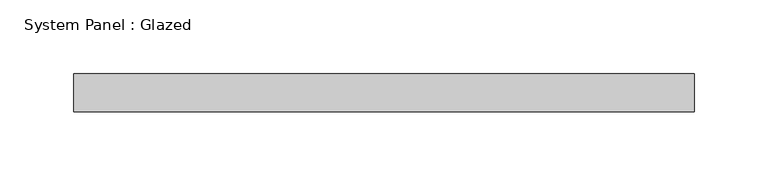
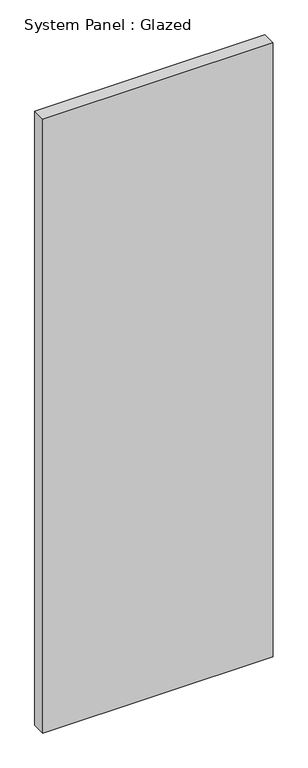
"""IFC4 building model written with IfcOpenShell, lengths in millimetres: plate geometry, System Panel : Glazed."""

from ifc_helpers import new_model, si_unit, origin, origin_with_axes, place, context, project, spatial, polyline, outline, extrude, source, transform, mapped, element, save


def system_panel_glazed_75a4b6fa(model_context):
    return source(origin(), model_context, "Body", "SweptSolid", [
        extrude(outline(polyline([(209.55, 19.05), (-209.55, 19.05), (-209.55, 44.45), (209.55, 44.45), (209.55, 19.05)])), origin_with_axes(), (0.0, 0.0, 1.0), 1181.1),
    ])


if __name__ == "__main__":
    model = new_model("IFC4")
    model_context = context("Model", 3, world=origin())
    ifc_project = project(units=[si_unit("LENGTHUNIT", "METRE", prefix="MILLI")], contexts=[model_context])
    site = spatial("IfcSite", under=ifc_project)
    building = spatial("IfcBuilding", under=site)
    placement = place(None, origin())
    system_panel_glazed_shape = system_panel_glazed_75a4b6fa(model_context)
    element("IfcPlate", 1, ObjectType="System Panel : Glazed", at=placement, inside=building, context=model_context, shape_type="MappedRepresentation", body=[
        mapped(system_panel_glazed_shape, transform((0.0, 0.0, 0.0), x_axis=(1.0, 0.0, 0.0), y_axis=(0.0, 1.0, 0.0), z_axis=(0.0, 0.0, 1.0))),
    ])
    save(model, "model.ifc")

# Revit data of these elements
# Type "System Panel : Glazed"
#   Construction Type Id = "GSP4R"
#   Analytic Construction = "1/8 in Pilkington single glazing"
#   Visual Light Transmittance = 0.9
#   Solar Heat Gain Coefficient = 0.86
#   Heat Transfer Coefficient (U) = 1.18115 BTU/(h·ft²·°F)
#   Define Thermal Properties by = 1
# Element 1 (IfcPlate, "System Panel : Glazed")
#   Materials on its faces: "Glass"
# Materials
#   "Glass": class "Glass", colour RGB 0 128 192, transparency 0.75, Description = "Soda Lime Glass", Cost = 0
